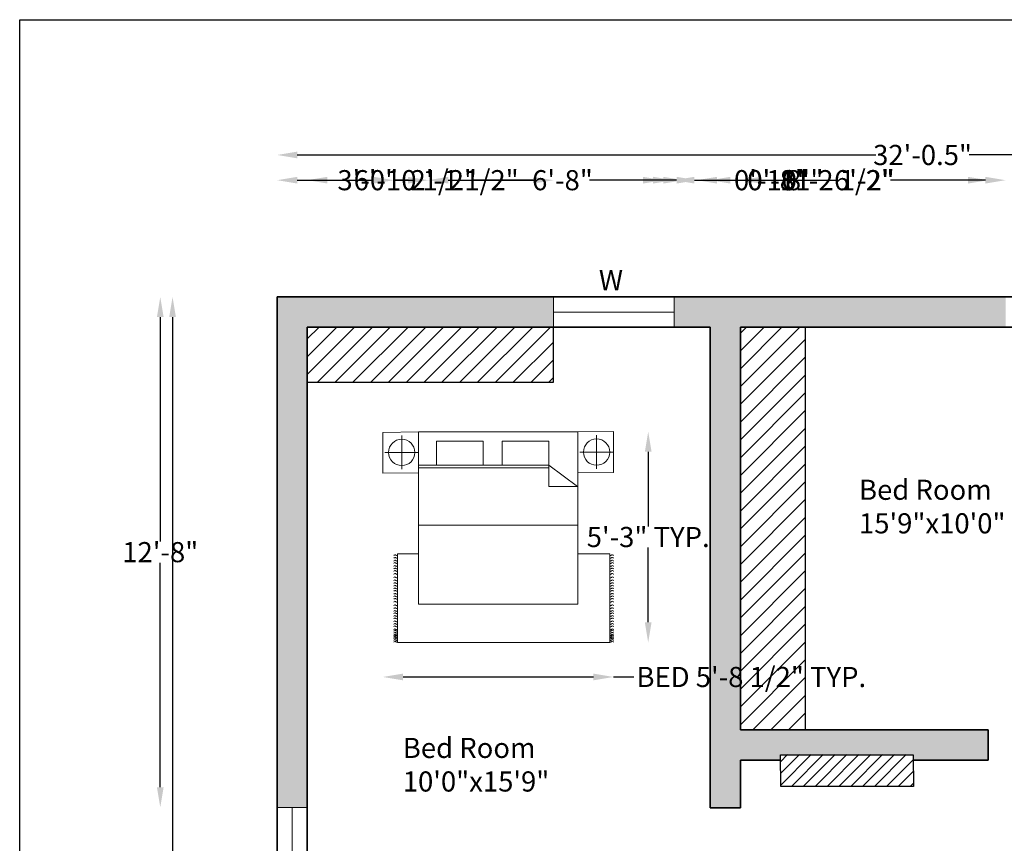
# Model space of a CAD drawing. Units: inches. Extents: x 1054 to 1577, y 4847 to 5610.
# Tile 4 of 5: x 1054 to 1347, y 5365 to 5610. Entities that reach past the tile are written whole.
import ezdxf

# ---------------------------------------------------------------- set-up
doc = ezdxf.new("R2010")
doc.units = ezdxf.units.IN
doc.header["$MEASUREMENT"] = 0
for name, color, linetype, lineweight in [('A-ANNO-DIMS', 2, 'Continuous', 18), ('A-ANNO-TEXT', 7, 'Continuous', 18), ('A-ANNO-TTLB', 7, 'Continuous', 25), ('A-AREA-IDEN', 7, 'Continuous', 18), ('A-FLOR-CASE', 7, 'Continuous', 25), ('A-FLOR-CASE-PATT', 252, 'Continuous', 13), ('A-GLAZ', 4, 'Continuous', 18), ('A-WALL', 7, 'Continuous', 35)]:
    doc.layers.add(name, color=color, linetype=linetype, lineweight=lineweight)
doc.layers.add('A-FURN', color=40, linetype='Continuous', lineweight=18, true_color=0xf8d731)
doc.layers.add('A-WALL-PATT', color=240, linetype='Continuous', lineweight=13, true_color=0xed1f24)
doc.styles.get("Standard").update_dxf_attribs({"font": 'arial.ttf'})
doc.dimstyles.get("Standard").update_dxf_attribs({"dimtxt": 6, "dimasz": 6, "dimexe": 0.18, "dimexo": 0.0625, "dimgap": 0.09, "dimtad": 0, "dimtih": 1, "dimtoh": 1, "dimdec": 1, "dimzin": 0, "dimdsep": 46, "dimlunit": 3, "dimtxsty": 'Standard', "dimcen": 0.09, "dimse1": 1, "dimse2": 1, "dimadec": 0, "dimazin": 0, "dimtfac": 1, "dimtdec": 1, "dimtofl": 0, "dimtmove": 0, "dimatfit": 3, "dimfxl": 1, "dimtolj": 1, "dimtzin": 0, "dimarcsym": 0})

# ---------------------------------------------------------------- blocks, each defined once
blk = doc.blocks.new('*D4')
at = {"layer": 'A-ANNO-DIMS', "color": 0, "lineweight": -2, "transparency": 16777216}
for p, q in [((1136.77, 5569.79), (1309.14, 5569.79)), ((1509.27, 5569.79), (1336.91, 5569.79))]:
    blk.add_line(p, q, dxfattribs=at)
at = {"layer": 'A-ANNO-DIMS', "color": 0, "transparency": 16777216}
for points in [[(1136.77, 5570.79), (1136.77, 5568.79), (1130.77, 5569.79)], [(1509.27, 5570.79), (1509.27, 5568.79), (1515.27, 5569.79)]]:
    blk.add_solid(points, dxfattribs=at)
at = {"layer": 'Defpoints', "color": 0, "transparency": 16777216}
for p in [(1515.27, 5569.79), (1130.77, 5527.48), (1515.27, 5527.48)]:
    blk.add_point(p, dxfattribs=at)
at = {"layer": 'A-ANNO-DIMS', "color": 0, "transparency": 16777216, "insert": (1323.02, 5569.79), "char_height": 6, "attachment_point": 5}
blk.add_mtext('\\A1;32\'-0.5"', dxfattribs=at)
blk = doc.blocks.new('*D5')
at = {"layer": 'A-ANNO-DIMS', "color": 0, "lineweight": -2, "transparency": 16777216}
for p, q in [((1099.63, 5521.48), (1099.63, 5260.62)), ((1099.63, 4993.48), (1099.63, 5254.34))]:
    blk.add_line(p, q, dxfattribs=at)
at = {"layer": 'A-ANNO-DIMS', "color": 0, "transparency": 16777216}
for points in [[(1098.63, 5521.48), (1100.63, 5521.48), (1099.63, 5527.48)], [(1098.63, 4993.48), (1100.63, 4993.48), (1099.63, 4987.48)]]:
    blk.add_solid(points, dxfattribs=at)
at = {"layer": 'Defpoints', "color": 0, "transparency": 16777216}
for p in [(1130.77, 5527.48), (1099.63, 4987.48), (1130.77, 4987.48)]:
    blk.add_point(p, dxfattribs=at)
at = {"layer": 'A-ANNO-DIMS', "color": 0, "transparency": 16777216, "insert": (1099.63, 5257.48), "char_height": 6, "attachment_point": 5}
blk.add_mtext("\\A1;45'", dxfattribs=at)
blk = doc.blocks.new('WINDOW-36IN')
for p, q in [((0, 9), (0, 0)), ((36, 9), (0, 9)), ((36, 0), (36, 9)), ((36, 4.5), (0, 4.5)), ((0, 0), (36, 0))]:
    blk.add_line(p, q)
blk = doc.blocks.new('BED-DOUBLE-WITH-TABLES')
for p, q in [((5.6, 61.62), (5.6, 51.56)), ((63.65, 61.72), (63.65, 51.66)), ((10.63, 56.59), (0.57, 56.59)), ((68.68, 56.69), (58.62, 56.69)), ((49.39, 52.82), (10.63, 52.82)), ((49.39, 52.82), (58, 46.47)), ((49.44, 52.82), (49.44, 46.47)), ((49.44, 52), (10.63, 52)), ((49.44, 46.47), (58, 46.47)), ((58.05, 34.96), (10.63, 34.96)), ((4.35, 0), (4.35, 26.37)), ((4.35, 26.37), (10.65, 26.37)), ((58.05, 26.37), (67.59, 26.37)), ((67.59, 26.37), (67.59, 0)), ((67.59, 0), (4.35, 0))]:
    blk.add_line(p, q)
for points in [[(0, 50.39), (10.63, 50.5), (10.63, 62.68), (0, 62.58)], [(58.05, 62.68), (58.05, 11.37), (10.63, 11.37), (10.63, 62.68)], [(58.05, 50.5), (68.68, 50.6), (68.68, 62.78), (58.05, 62.68)], [(29.88, 59.98), (29.88, 52.82), (15.98, 52.82), (15.98, 59.98)], [(49.44, 59.98), (49.44, 52.82), (35.55, 52.82), (35.55, 59.98)]]:
    blk.add_lwpolyline(points, close=True)
for centre in [(5.6, 56.59), (63.65, 56.69)]:
    blk.add_circle(centre, 3.92)
for points, knots in [([(3.23, 25.84), (3.32, 25.96), (3.52, 26.2), (3.86, 25.96), (4.14, 25.78), (4.29, 25.89), (4.35, 25.94)], [0, 0, 0, 0, 0.400747, 0.791423, 1.067667, 1.29709, 1.29709, 1.29709, 1.29709]), ([(3.23, 25.06), (3.32, 25.18), (3.52, 25.42), (3.86, 25.18), (4.14, 25.01), (4.29, 25.11), (4.35, 25.16)], [0, 0, 0, 0, 0.400747, 0.791423, 1.067667, 1.29709, 1.29709, 1.29709, 1.29709]), ([(3.23, 24.24), (3.32, 24.36), (3.52, 24.6), (3.86, 24.36), (4.14, 24.19), (4.29, 24.3), (4.35, 24.34)], [0, 0, 0, 0, 0.400747, 0.791423, 1.067667, 1.29709, 1.29709, 1.29709, 1.29709]), ([(3.23, 23.51), (3.32, 23.63), (3.52, 23.87), (3.86, 23.63), (4.14, 23.46), (4.29, 23.57), (4.35, 23.62)], [0, 0, 0, 0, 0.400747, 0.791423, 1.067667, 1.29709, 1.29709, 1.29709, 1.29709]), ([(68.71, 25.84), (68.61, 25.96), (68.42, 26.2), (68.08, 25.96), (67.8, 25.78), (67.65, 25.89), (67.58, 25.94)], [0, 0, 0, 0, 0.400747, 0.791423, 1.067667, 1.29709, 1.29709, 1.29709, 1.29709]), ([(68.71, 25.06), (68.61, 25.18), (68.42, 25.42), (68.08, 25.18), (67.8, 25.01), (67.65, 25.11), (67.58, 25.16)], [0, 0, 0, 0, 0.400747, 0.791423, 1.067667, 1.29709, 1.29709, 1.29709, 1.29709]), ([(68.71, 24.24), (68.61, 24.36), (68.42, 24.6), (68.08, 24.36), (67.8, 24.19), (67.65, 24.3), (67.58, 24.34)], [0, 0, 0, 0, 0.400747, 0.791423, 1.067667, 1.29709, 1.29709, 1.29709, 1.29709]), ([(68.71, 23.51), (68.61, 23.63), (68.42, 23.87), (68.08, 23.63), (67.8, 23.46), (67.65, 23.57), (67.58, 23.62)], [0, 0, 0, 0, 0.400747, 0.791423, 1.067667, 1.29709, 1.29709, 1.29709, 1.29709]), ([(3.23, 22.63), (3.32, 22.75), (3.52, 22.99), (3.86, 22.75), (4.14, 22.58), (4.29, 22.69), (4.35, 22.73)], [0, 0, 0, 0, 0.400747, 0.791423, 1.067667, 1.29709, 1.29709, 1.29709, 1.29709]), ([(3.23, 21.88), (3.32, 22), (3.52, 22.24), (3.86, 22), (4.14, 21.83), (4.29, 21.93), (4.35, 21.98)], [0, 0, 0, 0, 0.400747, 0.791423, 1.067667, 1.29709, 1.29709, 1.29709, 1.29709]), ([(3.23, 21.15), (3.32, 21.27), (3.52, 21.51), (3.86, 21.27), (4.14, 21.1), (4.29, 21.21), (4.35, 21.25)], [0, 0, 0, 0, 0.400747, 0.791423, 1.067667, 1.29709, 1.29709, 1.29709, 1.29709]), ([(3.23, 20.27), (3.32, 20.39), (3.52, 20.63), (3.86, 20.39), (4.14, 20.22), (4.29, 20.32), (4.35, 20.37)], [0, 0, 0, 0, 0.400747, 0.791423, 1.067667, 1.29709, 1.29709, 1.29709, 1.29709]), ([(68.71, 22.63), (68.61, 22.75), (68.42, 22.99), (68.08, 22.75), (67.8, 22.58), (67.65, 22.69), (67.58, 22.73)], [0, 0, 0, 0, 0.400747, 0.791423, 1.067667, 1.29709, 1.29709, 1.29709, 1.29709]), ([(68.71, 21.88), (68.61, 22), (68.42, 22.24), (68.08, 22), (67.8, 21.83), (67.65, 21.93), (67.58, 21.98)], [0, 0, 0, 0, 0.400747, 0.791423, 1.067667, 1.29709, 1.29709, 1.29709, 1.29709]), ([(68.71, 21.15), (68.61, 21.27), (68.42, 21.51), (68.08, 21.27), (67.8, 21.1), (67.65, 21.21), (67.58, 21.25)], [0, 0, 0, 0, 0.400747, 0.791423, 1.067667, 1.29709, 1.29709, 1.29709, 1.29709]), ([(68.71, 20.27), (68.61, 20.39), (68.42, 20.63), (68.08, 20.39), (67.8, 20.22), (67.65, 20.32), (67.58, 20.37)], [0, 0, 0, 0, 0.400747, 0.791423, 1.067667, 1.29709, 1.29709, 1.29709, 1.29709]), ([(3.23, 19.23), (3.32, 19.35), (3.52, 19.59), (3.86, 19.35), (4.14, 19.18), (4.29, 19.29), (4.35, 19.33)], [0, 0, 0, 0, 0.400747, 0.791423, 1.067667, 1.29709, 1.29709, 1.29709, 1.29709]), ([(3.23, 18.35), (3.32, 18.47), (3.52, 18.71), (3.86, 18.47), (4.14, 18.3), (4.29, 18.4), (4.35, 18.45)], [0, 0, 0, 0, 0.400747, 0.791423, 1.067667, 1.29709, 1.29709, 1.29709, 1.29709]), ([(3.23, 17.53), (3.32, 17.65), (3.52, 17.89), (3.86, 17.65), (4.14, 17.48), (4.29, 17.59), (4.35, 17.64)], [0, 0, 0, 0, 0.400747, 0.791423, 1.067667, 1.29709, 1.29709, 1.29709, 1.29709]), ([(68.71, 19.23), (68.61, 19.35), (68.42, 19.59), (68.08, 19.35), (67.8, 19.18), (67.65, 19.29), (67.58, 19.33)], [0, 0, 0, 0, 0.400747, 0.791423, 1.067667, 1.29709, 1.29709, 1.29709, 1.29709]), ([(68.71, 18.35), (68.61, 18.47), (68.42, 18.71), (68.08, 18.47), (67.8, 18.3), (67.65, 18.4), (67.58, 18.45)], [0, 0, 0, 0, 0.400747, 0.791423, 1.067667, 1.29709, 1.29709, 1.29709, 1.29709]), ([(68.71, 17.53), (68.61, 17.65), (68.42, 17.89), (68.08, 17.65), (67.8, 17.48), (67.65, 17.59), (67.58, 17.64)], [0, 0, 0, 0, 0.400747, 0.791423, 1.067667, 1.29709, 1.29709, 1.29709, 1.29709]), ([(3.23, 16.76), (3.32, 16.88), (3.52, 17.12), (3.86, 16.88), (4.14, 16.71), (4.29, 16.81), (4.35, 16.86)], [0, 0, 0, 0, 0.400747, 0.791423, 1.067667, 1.29709, 1.29709, 1.29709, 1.29709]), ([(3.23, 15.94), (3.32, 16.06), (3.52, 16.3), (3.86, 16.06), (4.14, 15.89), (4.29, 16), (4.35, 16.04)], [0, 0, 0, 0, 0.400747, 0.791423, 1.067667, 1.29709, 1.29709, 1.29709, 1.29709]), ([(3.23, 15.21), (3.32, 15.33), (3.52, 15.57), (3.86, 15.33), (4.14, 15.16), (4.29, 15.27), (4.35, 15.32)], [0, 0, 0, 0, 0.400747, 0.791423, 1.067667, 1.29709, 1.29709, 1.29709, 1.29709]), ([(68.71, 16.76), (68.61, 16.88), (68.42, 17.12), (68.08, 16.88), (67.8, 16.71), (67.65, 16.81), (67.58, 16.86)], [0, 0, 0, 0, 0.400747, 0.791423, 1.067667, 1.29709, 1.29709, 1.29709, 1.29709]), ([(68.71, 15.94), (68.61, 16.06), (68.42, 16.3), (68.08, 16.06), (67.8, 15.89), (67.65, 16), (67.58, 16.04)], [0, 0, 0, 0, 0.400747, 0.791423, 1.067667, 1.29709, 1.29709, 1.29709, 1.29709]), ([(68.71, 15.21), (68.61, 15.33), (68.42, 15.57), (68.08, 15.33), (67.8, 15.16), (67.65, 15.27), (67.58, 15.32)], [0, 0, 0, 0, 0.400747, 0.791423, 1.067667, 1.29709, 1.29709, 1.29709, 1.29709]), ([(3.23, 14.33), (3.32, 14.45), (3.52, 14.69), (3.86, 14.45), (4.14, 14.28), (4.29, 14.39), (4.35, 14.43)], [0, 0, 0, 0, 0.400747, 0.791423, 1.067667, 1.29709, 1.29709, 1.29709, 1.29709]), ([(3.23, 13.58), (3.32, 13.7), (3.52, 13.94), (3.86, 13.7), (4.14, 13.53), (4.29, 13.63), (4.35, 13.68)], [0, 0, 0, 0, 0.400747, 0.791423, 1.067667, 1.29709, 1.29709, 1.29709, 1.29709]), ([(3.23, 12.85), (3.32, 12.97), (3.52, 13.21), (3.86, 12.97), (4.14, 12.8), (4.29, 12.9), (4.35, 12.95)], [0, 0, 0, 0, 0.400747, 0.791423, 1.067667, 1.29709, 1.29709, 1.29709, 1.29709]), ([(3.23, 11.97), (3.32, 12.09), (3.52, 12.33), (3.86, 12.09), (4.14, 11.92), (4.29, 12.02), (4.35, 12.07)], [0, 0, 0, 0, 0.400747, 0.791423, 1.067667, 1.29709, 1.29709, 1.29709, 1.29709]), ([(68.71, 14.33), (68.61, 14.45), (68.42, 14.69), (68.08, 14.45), (67.8, 14.28), (67.65, 14.39), (67.58, 14.43)], [0, 0, 0, 0, 0.400747, 0.791423, 1.067667, 1.29709, 1.29709, 1.29709, 1.29709]), ([(68.71, 13.58), (68.61, 13.7), (68.42, 13.94), (68.08, 13.7), (67.8, 13.53), (67.65, 13.63), (67.58, 13.68)], [0, 0, 0, 0, 0.400747, 0.791423, 1.067667, 1.29709, 1.29709, 1.29709, 1.29709]), ([(68.71, 12.85), (68.61, 12.97), (68.42, 13.21), (68.08, 12.97), (67.8, 12.8), (67.65, 12.9), (67.58, 12.95)], [0, 0, 0, 0, 0.400747, 0.791423, 1.067667, 1.29709, 1.29709, 1.29709, 1.29709]), ([(68.71, 11.97), (68.61, 12.09), (68.42, 12.33), (68.08, 12.09), (67.8, 11.92), (67.65, 12.02), (67.58, 12.07)], [0, 0, 0, 0, 0.400747, 0.791423, 1.067667, 1.29709, 1.29709, 1.29709, 1.29709]), ([(3.23, 10.93), (3.32, 11.05), (3.52, 11.29), (3.86, 11.05), (4.14, 10.88), (4.29, 10.99), (4.35, 11.03)], [0, 0, 0, 0, 0.400747, 0.791423, 1.067667, 1.29709, 1.29709, 1.29709, 1.29709]), ([(3.23, 10.05), (3.32, 10.17), (3.52, 10.41), (3.86, 10.17), (4.14, 10), (4.29, 10.1), (4.35, 10.15)], [0, 0, 0, 0, 0.400747, 0.791423, 1.067667, 1.29709, 1.29709, 1.29709, 1.29709]), ([(3.23, 9.23), (3.32, 9.35), (3.52, 9.59), (3.86, 9.35), (4.14, 9.18), (4.29, 9.29), (4.35, 9.34)], [0, 0, 0, 0, 0.400747, 0.791423, 1.067667, 1.29709, 1.29709, 1.29709, 1.29709]), ([(3.23, 8.54), (3.32, 8.66), (3.52, 8.9), (3.86, 8.66), (4.14, 8.49), (4.29, 8.6), (4.35, 8.65)], [0, 0, 0, 0, 0.400747, 0.791423, 1.067667, 1.29709, 1.29709, 1.29709, 1.29709]), ([(68.71, 10.93), (68.61, 11.05), (68.42, 11.29), (68.08, 11.05), (67.8, 10.88), (67.65, 10.99), (67.58, 11.03)], [0, 0, 0, 0, 0.400747, 0.791423, 1.067667, 1.29709, 1.29709, 1.29709, 1.29709]), ([(68.71, 10.05), (68.61, 10.17), (68.42, 10.41), (68.08, 10.17), (67.8, 10), (67.65, 10.1), (67.58, 10.15)], [0, 0, 0, 0, 0.400747, 0.791423, 1.067667, 1.29709, 1.29709, 1.29709, 1.29709]), ([(68.71, 9.23), (68.61, 9.35), (68.42, 9.59), (68.08, 9.35), (67.8, 9.18), (67.65, 9.29), (67.58, 9.34)], [0, 0, 0, 0, 0.400747, 0.791423, 1.067667, 1.29709, 1.29709, 1.29709, 1.29709]), ([(68.71, 8.54), (68.61, 8.66), (68.42, 8.9), (68.08, 8.66), (67.8, 8.49), (67.65, 8.6), (67.58, 8.65)], [0, 0, 0, 0, 0.400747, 0.791423, 1.067667, 1.29709, 1.29709, 1.29709, 1.29709]), ([(3.23, 7.73), (3.32, 7.85), (3.52, 8.09), (3.86, 7.85), (4.14, 7.68), (4.29, 7.78), (4.35, 7.83)], [0, 0, 0, 0, 0.400747, 0.791423, 1.067667, 1.29709, 1.29709, 1.29709, 1.29709]), ([(3.23, 7), (3.32, 7.12), (3.52, 7.36), (3.86, 7.12), (4.14, 6.95), (4.29, 7.05), (4.35, 7.1)], [0, 0, 0, 0, 0.400747, 0.791423, 1.067667, 1.29709, 1.29709, 1.29709, 1.29709]), ([(3.23, 6.12), (3.32, 6.24), (3.52, 6.48), (3.86, 6.24), (4.14, 6.07), (4.29, 6.17), (4.35, 6.22)], [0, 0, 0, 0, 0.400747, 0.791423, 1.067667, 1.29709, 1.29709, 1.29709, 1.29709]), ([(68.71, 7.73), (68.61, 7.85), (68.42, 8.09), (68.08, 7.85), (67.8, 7.68), (67.65, 7.78), (67.58, 7.83)], [0, 0, 0, 0, 0.400747, 0.791423, 1.067667, 1.29709, 1.29709, 1.29709, 1.29709]), ([(68.71, 7), (68.61, 7.12), (68.42, 7.36), (68.08, 7.12), (67.8, 6.95), (67.65, 7.05), (67.58, 7.1)], [0, 0, 0, 0, 0.400747, 0.791423, 1.067667, 1.29709, 1.29709, 1.29709, 1.29709]), ([(68.71, 6.12), (68.61, 6.24), (68.42, 6.48), (68.08, 6.24), (67.8, 6.07), (67.65, 6.17), (67.58, 6.22)], [0, 0, 0, 0, 0.400747, 0.791423, 1.067667, 1.29709, 1.29709, 1.29709, 1.29709]), ([(3.23, 5.36), (3.32, 5.49), (3.52, 5.73), (3.86, 5.49), (4.14, 5.31), (4.29, 5.42), (4.35, 5.47)], [0, 0, 0, 0, 0.400747, 0.791423, 1.067667, 1.29709, 1.29709, 1.29709, 1.29709]), ([(3.23, 4.64), (3.32, 4.76), (3.52, 5), (3.86, 4.76), (4.14, 4.59), (4.29, 4.69), (4.35, 4.74)], [0, 0, 0, 0, 0.400747, 0.791423, 1.067667, 1.29709, 1.29709, 1.29709, 1.29709]), ([(3.23, 3.75), (3.32, 3.88), (3.52, 4.12), (3.86, 3.88), (4.14, 3.7), (4.29, 3.81), (4.35, 3.86)], [0, 0, 0, 0, 0.400747, 0.791423, 1.067667, 1.29709, 1.29709, 1.29709, 1.29709]), ([(3.23, 3.33), (3.32, 3.45), (3.51, 3.7), (3.86, 3.44), (4.14, 3.27), (4.29, 3.38), (4.35, 3.43)], [0, 0, 0, 0, 0.407265, 0.802015, 1.07826, 1.307683, 1.307683, 1.307683, 1.307683]), ([(3.23, 2.76), (3.32, 2.88), (3.52, 3.12), (3.86, 2.88), (4.14, 2.71), (4.29, 2.81), (4.35, 2.86)], [0, 0, 0, 0, 0.400747, 0.791423, 1.067667, 1.29709, 1.29709, 1.29709, 1.29709]), ([(68.71, 5.36), (68.61, 5.49), (68.42, 5.73), (68.08, 5.49), (67.8, 5.31), (67.65, 5.42), (67.58, 5.47)], [0, 0, 0, 0, 0.400747, 0.791423, 1.067667, 1.29709, 1.29709, 1.29709, 1.29709]), ([(68.71, 4.64), (68.61, 4.76), (68.42, 5), (68.08, 4.76), (67.8, 4.59), (67.66, 4.69), (67.59, 4.73)], [0, 0, 0, 0, 0.400747, 0.791423, 1.067667, 1.283686, 1.283686, 1.283686, 1.283686]), ([(68.71, 3.75), (68.61, 3.88), (68.42, 4.12), (68.08, 3.88), (67.8, 3.7), (67.66, 3.81), (67.59, 3.85)], [0, 0, 0, 0, 0.400747, 0.791423, 1.067667, 1.283686, 1.283686, 1.283686, 1.283686]), ([(68.71, 3.33), (68.61, 3.45), (68.42, 3.69), (68.08, 3.45), (67.8, 3.28), (67.66, 3.38), (67.59, 3.42)], [0, 0, 0, 0, 0.402903, 0.794912, 1.071156, 1.287177, 1.287177, 1.287177, 1.287177]), ([(68.71, 2.73), (68.61, 2.85), (68.42, 3.09), (68.08, 2.85), (67.8, 2.68), (67.66, 2.78), (67.59, 2.83)], [0, 0, 0, 0, 0.400747, 0.791423, 1.067667, 1.283686, 1.283686, 1.283686, 1.283686]), ([(3.23, 2.19), (3.32, 2.31), (3.52, 2.55), (3.86, 2.31), (4.14, 2.13), (4.29, 2.24), (4.35, 2.29)], [0, 0, 0, 0, 0.400747, 0.791423, 1.067667, 1.29709, 1.29709, 1.29709, 1.29709]), ([(3.23, 1.88), (3.32, 2), (3.52, 2.24), (3.86, 2), (4.14, 1.82), (4.29, 1.93), (4.35, 1.98)], [0, 0, 0, 0, 0.400747, 0.791423, 1.067667, 1.29709, 1.29709, 1.29709, 1.29709]), ([(3.23, 1.46), (3.32, 1.58), (3.52, 1.82), (3.86, 1.58), (4.14, 1.41), (4.29, 1.51), (4.35, 1.56)], [0, 0, 0, 0, 0.400747, 0.791423, 1.067667, 1.29709, 1.29709, 1.29709, 1.29709]), ([(3.23, 1.06), (3.32, 1.18), (3.52, 1.42), (3.86, 1.18), (4.14, 1.01), (4.29, 1.11), (4.35, 1.16)], [0, 0, 0, 0, 0.400747, 0.791423, 1.067667, 1.29709, 1.29709, 1.29709, 1.29709]), ([(3.23, 0.57), (3.32, 0.7), (3.52, 0.94), (3.86, 0.7), (4.14, 0.52), (4.29, 0.63), (4.35, 0.68)], [0, 0, 0, 0, 0.400747, 0.791423, 1.067667, 1.29709, 1.29709, 1.29709, 1.29709]), ([(3.23, 0.07), (3.32, 0.19), (3.52, 0.43), (3.86, 0.19), (4.14, 0.02), (4.29, 0.13), (4.35, 0.18)], [0, 0, 0, 0, 0.400747, 0.791423, 1.067667, 1.29709, 1.29709, 1.29709, 1.29709]), ([(68.71, 1.43), (68.61, 1.55), (68.42, 1.79), (68.08, 1.55), (67.8, 1.38), (67.65, 1.48), (67.58, 1.53)], [0, 0, 0, 0, 0.400747, 0.791423, 1.067667, 1.29709, 1.29709, 1.29709, 1.29709]), ([(68.71, 1.03), (68.61, 1.15), (68.42, 1.39), (68.08, 1.15), (67.8, 0.98), (67.65, 1.09), (67.58, 1.13)], [0, 0, 0, 0, 0.400747, 0.791423, 1.067667, 1.29709, 1.29709, 1.29709, 1.29709]), ([(68.71, 0.55), (68.61, 0.67), (68.42, 0.91), (68.08, 0.67), (67.8, 0.5), (67.65, 0.6), (67.58, 0.65)], [0, 0, 0, 0, 0.400747, 0.791423, 1.067667, 1.29709, 1.29709, 1.29709, 1.29709]), ([(68.71, 0.07), (68.61, 0.19), (68.42, 0.43), (68.08, 0.19), (67.8, 0.02), (67.65, 0.13), (67.58, 0.18)], [0, 0, 0, 0, 0.400747, 0.791423, 1.067667, 1.29709, 1.29709, 1.29709, 1.29709]), ([(68.71, 2.16), (68.61, 2.28), (68.42, 2.52), (68.08, 2.28), (67.8, 2.11), (67.66, 2.21), (67.59, 2.25)], [0, 0, 0, 0, 0.400747, 0.791423, 1.067667, 1.283686, 1.283686, 1.283686, 1.283686]), ([(68.71, 1.85), (68.61, 1.97), (68.42, 2.21), (68.08, 1.97), (67.8, 1.8), (67.66, 1.9), (67.59, 1.94)], [0, 0, 0, 0, 0.400747, 0.791423, 1.067667, 1.283686, 1.283686, 1.283686, 1.283686])]:
    blk.add_open_spline(points, degree=3, knots=knots)
blk = doc.blocks.new('*D12')
at = {"layer": 'A-ANNO-DIMS', "color": 0, "lineweight": -2, "transparency": 16777216}
for p, q in [((1168.28, 5414.26), (1224.99, 5414.26)), ((1230.99, 5414.26), (1236.99, 5414.26))]:
    blk.add_line(p, q, dxfattribs=at)
at = {"layer": 'A-ANNO-DIMS', "color": 0, "transparency": 16777216}
for points in [[(1168.28, 5415.26), (1168.28, 5413.26), (1162.28, 5414.26)], [(1224.99, 5415.26), (1224.99, 5413.26), (1230.99, 5414.26)]]:
    blk.add_solid(points, dxfattribs=at)
at = {"layer": 'Defpoints', "color": 0, "transparency": 16777216}
for p in [(1162.28, 5424.57), (1230.99, 5424.57), (1230.99, 5414.26)]:
    blk.add_point(p, dxfattribs=at)
at = {"layer": 'A-ANNO-DIMS', "color": 0, "transparency": 16777216, "insert": (1272.01, 5414.26), "char_height": 6, "attachment_point": 5}
blk.add_mtext('\\A1;BED 5\'-8 1/2" TYP.', dxfattribs=at)
blk = doc.blocks.new('*D13')
at = {"layer": 'A-ANNO-DIMS', "color": 0, "lineweight": -2, "transparency": 16777216}
for p, q in [((1241.3, 5481.35), (1241.3, 5459.11)), ((1241.3, 5430.57), (1241.3, 5452.8))]:
    blk.add_line(p, q, dxfattribs=at)
at = {"layer": 'A-ANNO-DIMS', "color": 0, "transparency": 16777216}
for points in [[(1240.3, 5481.35), (1242.3, 5481.35), (1241.3, 5487.35)], [(1240.3, 5430.57), (1242.3, 5430.57), (1241.3, 5424.57)]]:
    blk.add_solid(points, dxfattribs=at)
at = {"layer": 'Defpoints', "color": 0, "transparency": 16777216}
for p in [(1230.99, 5487.35), (1241.3, 5487.35), (1230.99, 5424.57)]:
    blk.add_point(p, dxfattribs=at)
at = {"layer": 'A-ANNO-DIMS', "color": 0, "transparency": 16777216, "insert": (1241.3, 5455.96), "char_height": 6, "attachment_point": 5}
blk.add_mtext('\\A1;5\'-3" TYP.', dxfattribs=at)
blk = doc.blocks.new('*D25')
at = {"layer": 'A-ANNO-DIMS', "color": 0, "lineweight": -2, "transparency": 16777216}
for p, q in [((1348.59, 4855.83), (1352.52, 4855.83)), ((1372.59, 4855.83), (1368.65, 4855.83))]:
    blk.add_line(p, q, dxfattribs=at)
at = {"layer": 'A-ANNO-DIMS', "color": 0, "transparency": 16777216}
for points in [[(1348.59, 4856.83), (1348.59, 4854.83), (1342.59, 4855.83)], [(1372.59, 4856.83), (1372.59, 4854.83), (1378.59, 4855.83)]]:
    blk.add_solid(points, dxfattribs=at)
at = {"layer": 'Defpoints', "color": 0, "transparency": 16777216}
for p in [(1342.59, 5389.48), (1378.59, 5389.48), (1378.59, 4855.83)]:
    blk.add_point(p, dxfattribs=at)
at = {"layer": 'A-ANNO-DIMS', "color": 0, "transparency": 16777216, "insert": (1360.59, 4855.83), "char_height": 6, "attachment_point": 5}
blk.add_mtext('\\A1;3\'-0"', dxfattribs=at)
blk = doc.blocks.new('*D29')
at = {"layer": 'A-ANNO-DIMS', "color": 0, "lineweight": -2, "transparency": 16777216}
for p, q in [((1136.77, 5562.28), (1154.52, 5562.28)), ((1207.08, 5562.28), (1189.33, 5562.28))]:
    blk.add_line(p, q, dxfattribs=at)
at = {"layer": 'A-ANNO-DIMS', "color": 0, "transparency": 16777216}
for points in [[(1136.77, 5563.28), (1136.77, 5561.28), (1130.77, 5562.28)], [(1207.08, 5563.28), (1207.08, 5561.28), (1213.08, 5562.28)]]:
    blk.add_solid(points, dxfattribs=at)
at = {"layer": 'Defpoints', "color": 0, "transparency": 16777216}
for p in [(1213.08, 5562.28), (1130.77, 5527.48), (1213.08, 5527.48)]:
    blk.add_point(p, dxfattribs=at)
at = {"layer": 'A-ANNO-DIMS', "color": 0, "transparency": 16777216, "insert": (1171.93, 5562.28), "char_height": 6, "attachment_point": 5}
blk.add_mtext('\\A1;6\'-10 1/2"', dxfattribs=at)
blk = doc.blocks.new('*D30')
at = {"layer": 'A-ANNO-DIMS', "color": 0, "lineweight": -2, "transparency": 16777216}
for p, q in [((1255.08, 5562.28), (1283.35, 5562.28)), ((1341.75, 5562.28), (1313.47, 5562.28))]:
    blk.add_line(p, q, dxfattribs=at)
at = {"layer": 'A-ANNO-DIMS', "color": 0, "transparency": 16777216}
for points in [[(1255.08, 5563.28), (1255.08, 5561.28), (1249.08, 5562.28)], [(1341.75, 5563.28), (1341.75, 5561.28), (1347.75, 5562.28)]]:
    blk.add_solid(points, dxfattribs=at)
at = {"layer": 'Defpoints', "color": 0, "transparency": 16777216}
for p in [(1347.75, 5562.28), (1249.08, 5527.48), (1347.75, 5527.48)]:
    blk.add_point(p, dxfattribs=at)
at = {"layer": 'A-ANNO-DIMS', "color": 0, "transparency": 16777216, "insert": (1298.41, 5562.28), "char_height": 6, "attachment_point": 5}
blk.add_mtext('\\A1;8\'-2 1/2"', dxfattribs=at)
blk = doc.blocks.new('*D35')
at = {"layer": 'A-ANNO-DIMS', "color": 0, "lineweight": -2, "transparency": 16777216}
for p, q in [((1095.97, 5521.48), (1095.97, 5454.6)), ((1095.97, 5381.41), (1095.97, 5448.29))]:
    blk.add_line(p, q, dxfattribs=at)
at = {"layer": 'A-ANNO-DIMS', "color": 0, "transparency": 16777216}
for points in [[(1094.97, 5521.48), (1096.97, 5521.48), (1095.97, 5527.48)], [(1094.97, 5381.41), (1096.97, 5381.41), (1095.97, 5375.41)]]:
    blk.add_solid(points, dxfattribs=at)
at = {"layer": 'Defpoints', "color": 0, "transparency": 16777216}
for p in [(1095.97, 5527.48), (1130.77, 5527.48), (1130.77, 5375.41)]:
    blk.add_point(p, dxfattribs=at)
at = {"layer": 'A-ANNO-DIMS', "color": 0, "transparency": 16777216, "insert": (1095.97, 5451.45), "char_height": 6, "attachment_point": 5}
blk.add_mtext('\\A1;12\'-8"', dxfattribs=at)
blk = doc.blocks.new('*D39')
at = {"layer": 'A-ANNO-DIMS', "color": 0, "lineweight": -2, "transparency": 16777216}
for p, q in [((1181.77, 5562.28), (1207.69, 5562.28)), ((1249.77, 5562.28), (1223.86, 5562.28))]:
    blk.add_line(p, q, dxfattribs=at)
at = {"layer": 'A-ANNO-DIMS', "color": 0, "transparency": 16777216}
for points in [[(1181.77, 5563.28), (1181.77, 5561.28), (1175.77, 5562.28)], [(1249.77, 5563.28), (1249.77, 5561.28), (1255.77, 5562.28)]]:
    blk.add_solid(points, dxfattribs=at)
at = {"layer": 'Defpoints', "color": 0, "transparency": 16777216}
for p in [(1255.77, 5562.28), (1175.77, 4996.48), (1255.77, 4996.48)]:
    blk.add_point(p, dxfattribs=at)
at = {"layer": 'A-ANNO-DIMS', "color": 0, "transparency": 16777216, "insert": (1215.77, 5562.28), "char_height": 6, "attachment_point": 5}
blk.add_mtext('\\A1;6\'-8"', dxfattribs=at)
blk = doc.blocks.new('*D40')
at = {"layer": 'A-ANNO-DIMS', "color": 0, "lineweight": -2, "transparency": 16777216}
for p, q in [((1145.77, 5562.28), (1149.71, 5562.28)), ((1169.77, 5562.28), (1165.84, 5562.28))]:
    blk.add_line(p, q, dxfattribs=at)
at = {"layer": 'A-ANNO-DIMS', "color": 0, "transparency": 16777216}
for points in [[(1145.77, 5563.28), (1145.77, 5561.28), (1139.77, 5562.28)], [(1169.77, 5563.28), (1169.77, 5561.28), (1175.77, 5562.28)]]:
    blk.add_solid(points, dxfattribs=at)
at = {"layer": 'Defpoints', "color": 0, "transparency": 16777216}
for p in [(1175.77, 5562.28), (1139.77, 4996.48), (1175.77, 4996.48)]:
    blk.add_point(p, dxfattribs=at)
at = {"layer": 'A-ANNO-DIMS', "color": 0, "transparency": 16777216, "insert": (1157.77, 5562.28), "char_height": 6, "attachment_point": 5}
blk.add_mtext('\\A1;3\'-0"', dxfattribs=at)
blk = doc.blocks.new('*D41')
at = {"layer": 'A-ANNO-DIMS', "color": 0, "lineweight": -2, "transparency": 16777216}
for p, q in [((1239.77, 5562.28), (1233.77, 5562.28)), ((1261.77, 5562.28), (1267.77, 5562.28))]:
    blk.add_line(p, q, dxfattribs=at)
at = {"layer": 'A-ANNO-DIMS', "color": 0, "transparency": 16777216}
for points in [[(1239.77, 5563.28), (1239.77, 5561.28), (1245.77, 5562.28)], [(1261.77, 5563.28), (1261.77, 5561.28), (1255.77, 5562.28)]]:
    blk.add_solid(points, dxfattribs=at)
at = {"layer": 'Defpoints', "color": 0, "transparency": 16777216}
for p in [(1255.77, 5562.28), (1245.77, 4996.48), (1255.77, 4996.48)]:
    blk.add_point(p, dxfattribs=at)
at = {"layer": 'A-ANNO-DIMS', "color": 0, "transparency": 16777216, "insert": (1278.17, 5562.28), "char_height": 6, "attachment_point": 5}
blk.add_mtext('\\A1;0\'-10"', dxfattribs=at)
blk = doc.blocks.new('*D43')
at = {"layer": 'A-ANNO-DIMS', "color": 0, "lineweight": -2, "transparency": 16777216}
for p, q in [((1550.07, 5389.48), (1550.07, 5395.48)), ((1550.07, 5395.48), (1556.07, 5395.48)), ((1550.07, 5381.26), (1550.07, 5383.48))]:
    blk.add_line(p, q, dxfattribs=at)
at = {"layer": 'A-ANNO-DIMS', "color": 0, "transparency": 16777216}
for points in [[(1549.07, 5383.48), (1551.07, 5383.48), (1550.07, 5389.48)], [(1549.07, 5381.26), (1551.07, 5381.26), (1550.07, 5375.26)]]:
    blk.add_solid(points, dxfattribs=at)
at = {"layer": 'Defpoints', "color": 0, "transparency": 16777216}
for p in [(1268.77, 5389.48), (1550.07, 5389.48), (1268.77, 5375.26)]:
    blk.add_point(p, dxfattribs=at)
at = {"layer": 'A-ANNO-DIMS', "color": 0, "transparency": 16777216, "insert": (1563.86, 5395.48), "char_height": 6, "attachment_point": 5}
blk.add_mtext('\\A1;1\'-2"', dxfattribs=at)
blk = doc.blocks.new('*D44')
at = {"layer": 'A-ANNO-DIMS', "color": 0, "lineweight": -2, "transparency": 16777216}
for p, q in [((1274.77, 5562.28), (1297.6, 5562.28)), ((1336.59, 5562.28), (1313.76, 5562.28))]:
    blk.add_line(p, q, dxfattribs=at)
at = {"layer": 'A-ANNO-DIMS', "color": 0, "transparency": 16777216}
for points in [[(1274.77, 5563.28), (1274.77, 5561.28), (1268.77, 5562.28)], [(1336.59, 5563.28), (1336.59, 5561.28), (1342.59, 5562.28)]]:
    blk.add_solid(points, dxfattribs=at)
at = {"layer": 'Defpoints', "color": 0, "transparency": 16777216}
for p in [(1342.59, 5562.28), (1268.77, 5398.48), (1342.59, 5398.48)]:
    blk.add_point(p, dxfattribs=at)
at = {"layer": 'A-ANNO-DIMS', "color": 0, "transparency": 16777216, "insert": (1305.68, 5562.28), "char_height": 6, "attachment_point": 5}
blk.add_mtext('\\A1;6\'-2"', dxfattribs=at)
blk = doc.blocks.new('*D47')
at = {"layer": 'A-ANNO-DIMS', "color": 0, "lineweight": -2, "transparency": 16777216}
for p, q in [((1242.78, 5562.28), (1236.78, 5562.28)), ((1265.77, 5562.28), (1271.77, 5562.28))]:
    blk.add_line(p, q, dxfattribs=at)
at = {"layer": 'A-ANNO-DIMS', "color": 0, "transparency": 16777216}
for points in [[(1242.78, 5563.28), (1242.78, 5561.28), (1248.78, 5562.28)], [(1265.77, 5563.28), (1265.77, 5561.28), (1259.77, 5562.28)]]:
    blk.add_solid(points, dxfattribs=at)
at = {"layer": 'Defpoints', "color": 0, "transparency": 16777216}
for p in [(1259.77, 5562.28), (1248.78, 5175.98), (1259.77, 5175.98)]:
    blk.add_point(p, dxfattribs=at)
at = {"layer": 'A-ANNO-DIMS', "color": 0, "transparency": 16777216, "insert": (1282.17, 5562.28), "char_height": 6, "attachment_point": 5}
blk.add_mtext('\\A1;0\'-11"', dxfattribs=at)
blk = doc.blocks.new('*D53')
at = {"layer": 'A-ANNO-DIMS', "color": 0, "lineweight": -2, "transparency": 16777216}
for p, q in [((1145.77, 5562.28), (1159.51, 5562.28)), ((1165.51, 5562.28), (1171.51, 5562.28))]:
    blk.add_line(p, q, dxfattribs=at)
at = {"layer": 'A-ANNO-DIMS', "color": 0, "transparency": 16777216}
for points in [[(1145.77, 5563.28), (1145.77, 5561.28), (1139.77, 5562.28)], [(1159.51, 5563.28), (1159.51, 5561.28), (1165.51, 5562.28)]]:
    blk.add_solid(points, dxfattribs=at)
at = {"layer": 'Defpoints', "color": 0, "transparency": 16777216}
for p in [(1165.51, 5562.28), (1165.51, 5077.04), (1139.77, 5075.48)]:
    blk.add_point(p, dxfattribs=at)
at = {"layer": 'A-ANNO-DIMS', "color": 0, "transparency": 16777216, "insert": (1186.62, 5562.28), "char_height": 6, "attachment_point": 5}
blk.add_mtext('\\A1;2\'-1 1/2"', dxfattribs=at)
blk = doc.blocks.new('*D54')
at = {"layer": 'A-ANNO-DIMS', "color": 0, "lineweight": -2, "transparency": 16777216}
for p, q in [((1245.84, 5562.28), (1239.84, 5562.28)), ((1265.77, 5562.28), (1271.77, 5562.28))]:
    blk.add_line(p, q, dxfattribs=at)
at = {"layer": 'A-ANNO-DIMS', "color": 0, "transparency": 16777216}
for points in [[(1245.84, 5563.28), (1245.84, 5561.28), (1251.84, 5562.28)], [(1265.77, 5563.28), (1265.77, 5561.28), (1259.77, 5562.28)]]:
    blk.add_solid(points, dxfattribs=at)
at = {"layer": 'Defpoints', "color": 0, "transparency": 16777216}
for p in [(1259.77, 5562.28), (1251.84, 5080.96), (1259.77, 5075.48)]:
    blk.add_point(p, dxfattribs=at)
at = {"layer": 'A-ANNO-DIMS', "color": 0, "transparency": 16777216, "insert": (1279.84, 5562.28), "char_height": 6, "attachment_point": 5}
blk.add_mtext('\\A1;0\'-8"', dxfattribs=at)

msp = doc.modelspace()

# ---------------------------------------------------------------- hatches: boundary and pattern name
at = {"layer": 'A-FLOR-CASE-PATT'}
h = msp.add_hatch(dxfattribs=at)
h.set_pattern_fill('ANSI31', color=256, scale=30)
h.paths.add_polyline_path([(1213.08, 5518.48), (1213.08, 5518.48), (1139.77, 5518.48), (1139.77, 5502.07), (1213.08, 5502.07)])
h.paths.add_polyline_path([(1288.09, 5518.48), (1268.77, 5518.48), (1268.77, 5398.48), (1288.09, 5398.48)])
h.paths.add_polyline_path([(1506.27, 5389.48), (1378.59, 5389.48), (1378.59, 5367.63), (1506.27, 5367.63)])
h = msp.add_hatch(dxfattribs=at)
h.set_pattern_fill('ANSI31', color=256, scale=20)
h.set_pattern_definition([(45, (0.0043, 0.008), (-1.767767, 1.767767), [])])
h.paths.add_polyline_path([(1320.19, 5391.11), (1280.67, 5391.11), (1280.8, 5381.65), (1320.31, 5381.65)])
at = {"layer": 'A-WALL-PATT'}
h = msp.add_hatch(color=256, dxfattribs=at)
h.dxf.hatch_style = 1
h.paths.add_polyline_path([(1213.08, 5527.48), (1130.77, 5527.48), (1130.77, 5375.41), (1139.77, 5375.41), (1139.77, 5518.48), (1213.08, 5518.48)])
h.paths.add_polyline_path([(1470.27, 5527.48), (1383.75, 5527.48), (1383.75, 5518.48), (1457.77, 5518.48), (1457.77, 5446.33), (1462.27, 5446.33), (1462.27, 5518.48), (1470.27, 5518.48)], flags=17)
h.paths.add_polyline_path([(1515.27, 5527.48), (1506.27, 5527.48), (1506.27, 5518.48), (1506.27, 5398.48), (1462.27, 5398.48), (1462.27, 5414.33), (1457.77, 5414.33), (1457.77, 5398.48), (1378.59, 5398.48), (1378.59, 5389.48), (1506.27, 5389.48), (1506.27, 5365.03), (1515.27, 5365.03)])
h.paths.add_polyline_path([(1515.27, 5329.03), (1506.27, 5329.03), (1506.27, 5255.01), (1515.27, 5255.01)])
h.paths.add_polyline_path([(1515.27, 5219.01), (1506.27, 5219.01), (1506.27, 5197.48), (1392.52, 5197.48), (1392.52, 5188.48), (1515.27, 5188.48)])
h.paths.add_polyline_path([(1344.52, 5197.48), (1268.77, 5197.48), (1268.77, 5215.14), (1259.77, 5215.14), (1259.77, 5175.98), (1248.78, 5175.98), (1248.78, 5171.48), (1259.77, 5171.48), (1259.77, 5075.48), (1139.77, 5075.48), (1139.77, 5124.09), (1130.77, 5124.09), (1130.77, 4987.48), (1268.77, 4987.48), (1268.77, 4996.48), (1139.77, 4996.48), (1139.77, 5066.48), (1175.77, 5066.48), (1268.77, 5066.48), (1268.77, 5188.48), (1344.52, 5188.48)])
h.paths.add_polyline_path([(1216.78, 5175.98), (1139.77, 5175.98), (1139.77, 5221.48), (1130.77, 5221.48), (1130.77, 5160.09), (1139.77, 5160.09), (1139.77, 5171.48), (1216.78, 5171.48)])
h.paths.add_polyline_path([(1268.77, 5339.26), (1259.77, 5339.26), (1259.77, 5329.48), (1247.44, 5329.48), (1247.44, 5324.98), (1259.77, 5324.98), (1259.77, 5276.98), (1139.77, 5276.98), (1139.77, 5281.9), (1130.77, 5281.9), (1130.77, 5257.48), (1139.77, 5257.48), (1139.77, 5267.98), (1259.77, 5267.98), (1259.77, 5251.14), (1268.77, 5251.14)])
h.paths.add_polyline_path([(1139.77, 5339.41), (1130.77, 5339.41), (1130.77, 5317.9), (1139.77, 5317.9), (1139.77, 5324.98), (1215.44, 5324.98), (1215.44, 5329.48), (1139.77, 5329.48)])
h.paths.add_polyline_path([(1280.67, 5389.48), (1280.67, 5391.1), (1320.18, 5391.1), (1320.18, 5389.48), (1342.59, 5389.48), (1342.59, 5398.48), (1268.77, 5398.48), (1268.77, 5518.48), (1347.75, 5518.48), (1347.75, 5527.48), (1249.08, 5527.48), (1249.08, 5518.48), (1259.77, 5518.48), (1259.77, 5375.26), (1268.77, 5375.26), (1268.77, 5389.48)])

# ---------------------------------------------------------------- linework, layer by layer
at = {"layer": 'A-ANNO-TTLB'}
msp.add_lwpolyline([(1054.1, 5610.1), (1577.31, 5610.1), (1577.31, 4927.21), (1054.1, 4927.21)], close=True, dxfattribs=at)
at = {"layer": 'A-FLOR-CASE'}
for p, q in [((1213.08, 5502.07), (1213.08, 5518.48)), ((1268.77, 5518.48), (1288.09, 5518.48)), ((1288.09, 5518.48), (1288.09, 5398.48)), ((1139.77, 5502.07), (1213.08, 5502.07))]:
    msp.add_line(p, q, dxfattribs=at)
msp.add_lwpolyline([(1280.67, 5391.1), (1320.18, 5391.1), (1320.31, 5381.65), (1280.8, 5381.65)], close=True, dxfattribs=at)
at = {"layer": 'A-GLAZ'}
for p, q in [((1213.08, 5518.48), (1213.08, 5527.48)), ((1213.08, 5527.48), (1249.08, 5527.48)), ((1249.08, 5527.48), (1249.08, 5518.48)), ((1213.08, 5522.98), (1249.08, 5522.98)), ((1249.08, 5518.48), (1213.08, 5518.48))]:
    msp.add_line(p, q, dxfattribs=at)
at = {"layer": 'A-WALL'}
for p, q in [((1130.77, 5527.48), (1515.27, 5527.48)), ((1130.77, 5527.48), (1130.77, 4987.48)), ((1139.77, 5518.48), (1139.77, 5329.48)), ((1139.77, 5518.48), (1259.77, 5518.48)), ((1259.77, 5518.48), (1259.77, 5375.26)), ((1268.77, 5518.48), (1268.77, 5398.48)), ((1268.77, 5518.48), (1457.77, 5518.48)), ((1268.77, 5398.48), (1342.59, 5398.48)), ((1342.59, 5398.48), (1342.59, 5389.48)), ((1268.77, 5389.48), (1280.67, 5389.48)), ((1268.77, 5389.48), (1268.77, 5375.26)), ((1320.18, 5389.48), (1342.59, 5389.48)), ((1259.77, 5375.26), (1268.77, 5375.26))]:
    msp.add_line(p, q, dxfattribs=at)

# ---------------------------------------------------------------- block references
at = {"layer": 'A-FURN'}
msp.add_blockref('BED-DOUBLE-WITH-TABLES', (1162.28, 5424.57), dxfattribs=at)
at = {"layer": 'A-GLAZ', "rotation": 89.99999999999471}
msp.add_blockref('WINDOW-36IN', (1139.77, 5339.41), dxfattribs=at)

# ---------------------------------------------------------------- texts
at = {"layer": 'A-ANNO-TEXT', "insert": (1226.61, 5535.51), "char_height": 6, "attachment_point": 1}
msp.add_mtext_dynamic_manual_height_columns('W', width=11.4277, gutter_width=30, heights=[0], dxfattribs=at)
at = {"layer": 'A-AREA-IDEN', "char_height": 6, "attachment_point": 1}
for s, width, insert in [('Bed Room\\P15\'9"x10\'0"', 53.797, (1304.09, 5473.04)), ('Bed Room\\P10\'0"x15\'9"', 62.2184, (1168.2, 5396.12))]:
    msp.add_mtext_dynamic_manual_height_columns(s, width=width, gutter_width=30, heights=[0], dxfattribs=dict(at, insert=insert))

# ---------------------------------------------------------------- dimensions: what is measured, and where the dimension line sits
at = {"layer": 'A-ANNO-DIMS'}
for base, p1, p2, override, picture, middle in [((1515.27, 5569.79), (1130.77, 5527.48), (1515.27, 5527.48), {"dimclrd": 0, "dimclre": 0, "dimclrt": 0}, '*D4', (1323.02, 5569.79)), ((1213.08, 5562.28), (1130.77, 5527.48), (1213.08, 5527.48), {"dimdec": 1, "dimlfac": 1, "dimrnd": 0, "dimzin": 1, "dimdsep": 46, "dimlunit": 4, "dimfrac": 2}, '*D29', (1171.93, 5562.28)), ((1165.51, 5562.28), (1139.77, 5075.48), (1165.51, 5077.04), {"dimdec": 1, "dimlfac": 1, "dimrnd": 0, "dimzin": 1, "dimdsep": 46, "dimlunit": 4, "dimfrac": 2}, '*D53', (1186.62, 5562.28)), ((1347.75, 5562.28), (1249.08, 5527.48), (1347.75, 5527.48), {"dimdec": 1, "dimlfac": 1, "dimrnd": 0, "dimzin": 1, "dimdsep": 46, "dimlunit": 4, "dimfrac": 2}, '*D30', (1298.41, 5562.28)), ((1175.77, 5562.28), (1139.77, 4996.48), (1175.77, 4996.48), {"dimdec": 1, "dimlfac": 1, "dimrnd": 0, "dimzin": 1, "dimdsep": 46, "dimlunit": 4, "dimfrac": 2}, '*D40', (1157.77, 5562.28)), ((1255.77, 5562.28), (1175.77, 4996.48), (1255.77, 4996.48), {"dimdec": 1, "dimlfac": 1, "dimrnd": 0, "dimzin": 1, "dimdsep": 46, "dimlunit": 4, "dimfrac": 2}, '*D39', (1215.77, 5562.28)), ((1255.77, 5562.28), (1245.77, 4996.48), (1255.77, 4996.48), {"dimdec": 1, "dimlfac": 1, "dimrnd": 0, "dimzin": 1, "dimdsep": 46, "dimlunit": 4, "dimfrac": 2}, '*D41', (1278.17, 5562.28)), ((1259.77, 5562.28), (1248.78, 5175.98), (1259.77, 5175.98), {"dimdec": 1, "dimlfac": 1, "dimrnd": 0, "dimzin": 1, "dimdsep": 46, "dimlunit": 4, "dimfrac": 2}, '*D47', (1282.17, 5562.28)), ((1259.77, 5562.28), (1251.84, 5080.96), (1259.77, 5075.48), {"dimdec": 1, "dimlfac": 1, "dimrnd": 0, "dimzin": 1, "dimdsep": 46, "dimlunit": 4, "dimfrac": 2}, '*D54', (1279.84, 5562.28)), ((1342.59, 5562.28), (1268.77, 5398.48), (1342.59, 5398.48), {"dimdec": 1, "dimlfac": 1, "dimrnd": 0, "dimzin": 1, "dimdsep": 46, "dimlunit": 4, "dimfrac": 2}, '*D44', (1305.68, 5562.28)), ((1378.59, 4855.83), (1342.59, 5389.48), (1378.59, 5389.48), {"dimdec": 1, "dimlfac": 1, "dimrnd": 0, "dimzin": 1, "dimdsep": 46, "dimlunit": 4, "dimfrac": 2}, '*D25', (1360.59, 4855.83))]:
    dim = msp.add_linear_dim(base=base, p1=p1, p2=p2, dimstyle='Standard', override=override, dxfattribs=at)
    dim.commit()
    dim.dimension.update_dxf_attribs({"geometry": picture, "text_midpoint": middle})
for base, p1, p2, override, picture, middle in [((1095.97, 5527.48), (1130.77, 5375.41), (1130.77, 5527.48), {"dimdec": 1, "dimlfac": 1, "dimrnd": 0, "dimzin": 1, "dimdsep": 46, "dimlunit": 4, "dimfrac": 2}, '*D35', (1095.97, 5451.45)), ((1099.63, 4987.48), (1130.77, 5527.48), (1130.77, 4987.48), {"dimclrd": 0, "dimclre": 0, "dimclrt": 0}, '*D5', (1099.63, 5257.48)), ((1550.07, 5389.48), (1268.77, 5375.26), (1268.77, 5389.48), {"dimdec": 1, "dimlfac": 1, "dimrnd": 0, "dimzin": 1, "dimdsep": 46, "dimlunit": 4, "dimfrac": 2}, '*D43', (1563.86, 5395.48))]:
    dim = msp.add_linear_dim(base=base, p1=p1, p2=p2, angle=90, dimstyle='Standard', override=override, dxfattribs=at)
    dim.commit()
    dim.dimension.update_dxf_attribs({"geometry": picture, "text_midpoint": middle})
dim = msp.add_linear_dim(base=(1241.3, 5487.35), p1=(1230.99, 5424.57), p2=(1230.99, 5487.35), angle=90, text='<> TYP.', dimstyle='Standard', override={"dimdec": 1, "dimlfac": 1, "dimrnd": 0, "dimzin": 1, "dimdsep": 46, "dimlunit": 4, "dimfrac": 2}, dxfattribs=at)
dim.commit()
dim.dimension.update_dxf_attribs({"geometry": '*D13', "text_midpoint": (1241.3, 5455.96)})
dim = msp.add_linear_dim(base=(1230.99, 5414.26), p1=(1162.28, 5424.57), p2=(1230.99, 5424.57), text='BED <> TYP.', dimstyle='Standard', override={"dimdec": 1, "dimlfac": 1, "dimrnd": 0, "dimzin": 1, "dimdsep": 46, "dimlunit": 4, "dimfrac": 2}, dxfattribs=at)
dim.commit()
dim.dimension.update_dxf_attribs({"geometry": '*D12', "text_midpoint": (1272.01, 5414.26)})

doc.saveas('drawing.dxf')
